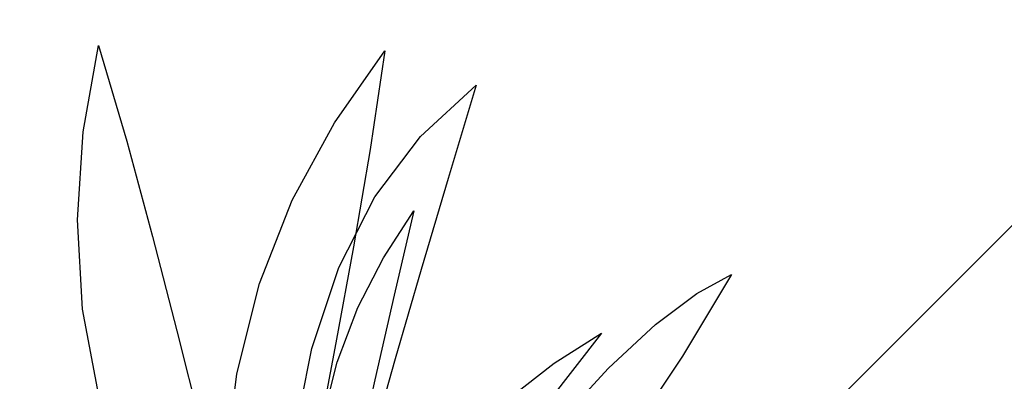
# Model space of a CAD drawing. Units: inches. Extents: x 3590 to 5167, y 65 to 1917.
# Tile 53 of 100: x 4947.17 to 4967.82, y 1530.53 to 1538.11. Entities that reach past the tile are written whole.
import ezdxf

# ---------------------------------------------------------------- set-up
doc = ezdxf.new("R2010")
doc.units = ezdxf.units.IN
doc.layers.add('A-FLOR-PATT', color=8, linetype='Continuous', lineweight=13)
doc.layers.add('L-PLNT', color=94, linetype='Continuous', lineweight=18)
doc.layers.add('DIENHOA', color=3, linetype='Continuous')

# ---------------------------------------------------------------- blocks, each defined once
blk = doc.blocks.new('Cay03_mb')
at = {"layer": 'DIENHOA'}
for p, q in [((118.58, 555.3), (166.15, 599.14)), ((166.15, 599.14), (142.15, 519.35)), ((79.49, 503.68), (118.58, 555.3)), ((142.15, 519.35), (118.96, 441.66)), ((48.56, 443.58), (79.49, 503.68)), ((25.49, 374.33), (48.56, 443.58)), ((118.96, 441.66), (96.72, 365.58)), ((9.94, 295.25), (25.49, 374.33)), ((96.72, 365.58), (75.6, 290.61))]:
    blk.add_line(p, q, dxfattribs=at)
for points in [[(23.69, -5.44), (-41, 82.2), (-91.83, 167.08), (-129.72, 249.45), (-155.55, 329.59), (-170.25, 407.76), (-174.71, 484.23), (-169.84, 559.26), (-156.54, 633.12)], [(-156.54, 633.12), (-132.46, 551.33), (-110.51, 470.02), (-89.84, 389.22), (-69.62, 308.98), (-48.99, 229.35), (-27.13, 150.38), (-3.18, 72.1), (23.69, -5.44)], [(-16.39, -26.73), (-38.34, 79.96), (-48.88, 178.33), (-48.7, 269), (-38.53, 352.58), (-19.08, 429.71), (8.95, 500.99), (44.86, 567.06), (87.92, 628.52)], [(87.92, 628.52), (75.46, 544.18), (61.27, 461.15), (46.13, 379.14), (30.83, 297.82), (16.14, 216.89), (2.85, 136.03), (-8.25, 54.92), (-16.39, -26.73)], [(23.69, -5.44), (19.84, 92.99), (20.28, 176.97), (25.02, 248.55), (34.03, 309.77), (47.33, 362.68), (64.91, 409.31), (86.75, 451.72), (112.87, 491.95)], [(112.87, 491.95), (95.99, 419.69), (79.46, 347.37), (63.92, 276.46), (50.01, 208.43), (38.38, 144.75), (29.69, 86.9), (24.57, 36.35), (23.69, -5.44)], [(384.28, 437.45), (342.25, 367.83), (298.14, 301.71), (252.56, 239.37), (206.11, 181.11), (159.39, 127.21), (113.01, 77.96), (67.57, 33.64), (23.69, -5.44)], [(23.69, -5.44), (79.88, 91.71), (134.12, 176.21), (185.81, 248.4), (234.31, 308.65), (279.02, 357.33), (319.33, 394.78), (354.62, 421.37), (384.28, 437.45)], [(273.24, 387.35), (227.6, 328.83), (182.25, 270.12), (138.39, 212.28), (97.23, 156.36), (59.96, 103.43), (27.8, 54.57), (1.94, 10.82), (-16.39, -26.73)], [(-16.39, -26.73), (21.41, 64.22), (57.05, 140.27), (91.37, 203.26), (125.24, 255.05), (159.51, 297.5), (195.03, 332.46), (232.65, 361.79), (273.24, 387.35)]]:
    blk.add_lwpolyline(points, dxfattribs=at)

msp = doc.modelspace()

# ---------------------------------------------------------------- hatches: boundary and pattern name
at = {"layer": 'A-FLOR-PATT', "transparency": 33554687}
h = msp.add_hatch(dxfattribs=at)
h.set_pattern_fill('AR-HBONE', color=256, scale=0.2)
h.set_pattern_definition([(45, (-588.972, 0), (0, 28.73682), [60.96, -20.32]), (135, (-574.604, 14.368), (3e-15, 28.73682), [60.96, -20.32])])
h.paths.add_polyline_path([(5071.274, 1796.999), (4933.274, 1796.999), (4933.274, 1753.999), (4962.774, 1753.999, -0.414214), (4928.774, 1719.999), (4933.274, 1718.999), (4933.274, 1334.999), (5071.274, 1334.999)])
h.paths.add_polyline_path([(4951.78, 1521.077), (4951.715, 1521.04), (4951.563, 1520.895)], flags=16)
h.paths.add_polyline_path([(4952.267, 1521.376), (4952.198, 1521.371), (4952.198, 1521.356)], flags=0)
h.paths.add_polyline_path([(4967.051, 1529.728), (4965.231, 1528.694), (4963.411, 1527.714), (4961.756, 1526.851), (4963.589, 1527.449), (4964.036, 1527.478), (4962.975, 1527.249), (4961.76, 1526.852), (4959.792, 1525.834), (4958.005, 1524.895), (4956.24, 1523.93), (4954.504, 1522.919), (4954.129, 1522.682), (4953.361, 1521.997), (4953.366, 1521.998), (4953.605, 1522.064), (4955.106, 1522.761), (4956.921, 1523.434), (4958.678, 1523.915), (4960.358, 1524.2), (4961.945, 1524.286), (4964.171, 1524.108), (4965.958, 1523.309), (4963.863, 1522.976), (4965.187, 1522.499), (4963.366, 1522.497), (4961.545, 1522.487), (4959.764, 1522.461), (4958.304, 1522.419), (4957.974, 1522.388), (4956.307, 1522.232), (4954.718, 1522.071), (4953.251, 1521.899), (4953.525, 1521.623), (4954.331, 1521.379), (4956.243, 1521.23), (4958.039, 1520.93), (4959.684, 1520.483), (4961.16, 1519.896), (4963.107, 1518.8), (4964.393, 1517.325), (4962.973, 1517.726), (4964.558, 1516.661), (4965.407, 1515.708), (4963.507, 1516.322), (4961.68, 1517.005), (4959.935, 1517.745), (4958.282, 1518.528), (4956.732, 1519.343), (4955.295, 1520.175), (4954.672, 1520.572), (4954.513, 1520.627), (4955.658, 1519.318), (4956.703, 1517.982), (4957.644, 1516.647), (4958.485, 1515.334), (4959.55, 1513.524), (4960.438, 1511.769), (4958.841, 1513.62), (4957.452, 1515.325), (4955.819, 1517.459), (4956.665, 1515.448), (4957.111, 1513.923), (4957.447, 1511.714), (4957.076, 1509.793), (4956.538, 1511.11), (4955.992, 1512.569), (4955.444, 1514.125), (4954.898, 1515.735), (4954.357, 1517.356), (4953.824, 1518.943), (4953.305, 1520.452), (4953.065, 1521.116), (4952.971, 1521.146), (4952.949, 1521.086), (4952.73, 1520.199), (4953.37, 1518.024), (4953.757, 1516.373), (4954.051, 1514.765), (4954.264, 1513.221), (4954.471, 1511.131), (4954.497, 1510.402), (4954.409, 1511.76), (4954.264, 1513.221), (4954.051, 1514.765), (4953.757, 1516.373), (4953.37, 1518.024), (4952.877, 1519.698), (4952.716, 1520.141), (4952.533, 1519.059), (4952.374, 1517.789), (4952.219, 1516.312), (4952.046, 1514.6), (4951.833, 1512.626), (4951.557, 1510.363), (4951.203, 1512.168), (4950.852, 1514.339), (4950.985, 1516.376), (4951.66, 1518.286), (4952.593, 1520.481), (4952.357, 1521.13), (4951.855, 1520.328), (4950.839, 1518.908), (4949.777, 1517.587), (4948.916, 1516.617), (4948.111, 1515.256), (4947.089, 1513.554), (4945.889, 1511.615), (4946.326, 1513.402), (4946.562, 1514.249), (4945.528, 1513.327), (4944.581, 1512.531), (4946.018, 1514.508), (4947.204, 1516.048), (4947.893, 1517.313), (4949.307, 1518.764), (4950.414, 1519.767), (4950.451, 1519.806), (4952.267, 1521.376), (4951.645, 1521.493), (4950.404, 1521.18), (4948.044, 1520.359), (4946.119, 1519.452), (4944.572, 1518.475), (4943.35, 1517.443), (4941.997, 1515.92), (4941.661, 1515.275), (4942.813, 1516.99), (4944.572, 1518.475), (4946.119, 1519.452), (4948.044, 1520.359), (4950.404, 1521.18), (4951.645, 1521.493), (4949.647, 1521.868), (4948.6, 1521.756), (4947.126, 1521.57), (4945.42, 1521.348), (4943.45, 1521.105), (4941.183, 1520.856), (4942.86, 1521.613), (4943.873, 1522.03), (4942.952, 1521.909), (4941.41, 1521.485), (4939.543, 1520.67), (4938.968, 1520.226), (4940.733, 1521.299), (4942.952, 1521.909), (4943.702, 1522.008), (4945.894, 1522.7), (4947.565, 1522.714), (4948.921, 1522.566), (4951.131, 1522.183), (4950.971, 1522.297), (4948.129, 1523.006), (4946.035, 1523.707), (4944.232, 1524.521), (4942.707, 1525.461), (4941.444, 1526.537), (4940.43, 1527.761), (4939.649, 1529.143), (4941.421, 1528.122), (4943.147, 1527.132), (4944.841, 1526.175), (4946.514, 1525.25), (4948.179, 1524.359), (4948.365, 1524.263), (4946.475, 1526.045), (4945.181, 1527.54), (4944.19, 1529.033), (4943.496, 1530.54), (4943.278, 1531.36), (4942.498, 1531.919), (4943.114, 1531.762), (4942.959, 1533.659), (4944.14, 1531.989), (4944.612, 1531.323), (4946.202, 1530.463), (4947.486, 1529.509), (4948.79, 1528.226), (4950.368, 1526.237), (4949.485, 1528.155), (4948.851, 1530.123), (4948.491, 1532.041), (4948.381, 1533.918), (4948.501, 1535.76), (4948.827, 1537.573), (4949.418, 1535.565), (4949.957, 1533.569), (4950.464, 1531.586), (4950.961, 1529.617), (4951.391, 1527.954), (4951.724, 1530.687), (4952.201, 1532.58), (4952.889, 1534.33), (4953.77, 1535.951), (4954.827, 1537.46), (4954.521, 1535.39), (4954.273, 1533.937), (4955.58, 1535.663), (4956.748, 1536.739), (4956.159, 1534.78), (4955.589, 1532.873), (4955.043, 1531.006), (4954.525, 1529.166), (4954.038, 1527.341), (4953.638, 1525.733), (4953.611, 1525.586), (4953.398, 1524.166), (4953.382, 1524.009), (4954.07, 1525.476), (4954.912, 1527.022), (4956.136, 1528.894), (4957.847, 1530.577), (4959.376, 1531.54), (4958.256, 1530.104), (4957.143, 1528.663), (4956.066, 1527.243), (4955.056, 1525.871), (4954.141, 1524.571), (4953.352, 1523.372), (4953.311, 1523.303), (4953.273, 1522.925), (4953.261, 1522.382), (4954.103, 1523.373), (4954.63, 1524.284), (4955.961, 1526.358), (4957.23, 1528.13), (4958.421, 1529.609), (4960.037, 1531.368), (4961.374, 1532.375), (4962.101, 1532.77), (4961.07, 1531.061), (4959.987, 1529.438), (4958.869, 1527.908), (4958.15, 1527.007), (4959.803, 1528.003), (4961.589, 1528.793), (4963.391, 1529.328), (4965.211, 1529.632)], flags=16)
h.paths.add_polyline_path([(4962.944, 1523.182), (4961.107, 1523.422), (4960.392, 1523.362), (4962.35, 1523.331)], flags=0)
h.paths.add_polyline_path([(5049.541, 1584.551), (5049.476, 1584.515), (5049.325, 1584.37)], flags=16)
h.paths.add_polyline_path([(5050.028, 1584.851), (5049.959, 1584.845), (5049.959, 1584.83)], flags=0)
h.paths.add_polyline_path([(5042.333, 1581.949), (5043.88, 1582.926), (5045.806, 1583.833), (5048.165, 1584.654), (5049.406, 1584.967), (5047.408, 1585.342), (5046.361, 1585.231), (5044.888, 1585.044), (5043.181, 1584.822), (5041.211, 1584.579), (5038.944, 1584.33), (5040.622, 1585.087), (5041.634, 1585.504), (5040.713, 1585.383), (5039.171, 1584.959), (5037.304, 1584.144), (5036.729, 1583.7), (5038.494, 1584.773), (5040.713, 1585.383), (5041.463, 1585.482), (5043.655, 1586.174), (5045.326, 1586.188), (5046.682, 1586.04), (5048.893, 1585.657), (5048.732, 1585.771), (5045.891, 1586.48), (5043.796, 1587.181), (5041.994, 1587.996), (5040.468, 1588.935), (5039.205, 1590.011), (5038.191, 1591.235), (5037.41, 1592.617), (5039.182, 1591.596), (5040.909, 1590.607), (5042.602, 1589.649), (5044.275, 1588.724), (5045.94, 1587.833), (5046.126, 1587.738), (5044.237, 1589.519), (5042.942, 1591.015), (5041.952, 1592.508), (5041.257, 1594.014), (5041.039, 1594.834), (5040.26, 1595.393), (5040.875, 1595.237), (5040.721, 1597.133), (5041.901, 1595.463), (5042.373, 1594.798), (5043.963, 1593.938), (5045.247, 1592.983), (5046.552, 1591.701), (5048.129, 1589.712), (5047.247, 1591.63), (5046.613, 1593.597), (5046.252, 1595.515), (5046.142, 1597.392), (5046.262, 1599.234), (5046.588, 1601.047), (5047.179, 1599.039), (5047.718, 1597.043), (5048.225, 1595.06), (5048.722, 1593.091), (5049.152, 1591.429), (5049.485, 1594.161), (5049.962, 1596.054), (5050.65, 1597.804), (5051.532, 1599.425), (5052.589, 1600.934), (5052.283, 1598.864), (5052.034, 1597.411), (5053.341, 1599.137), (5054.509, 1600.213), (5053.92, 1598.254), (5053.35, 1596.348), (5052.805, 1594.48), (5052.286, 1592.64), (5051.799, 1590.815), (5051.4, 1589.207), (5051.373, 1589.06), (5051.159, 1587.64), (5051.143, 1587.483), (5051.831, 1588.95), (5052.673, 1590.496), (5053.898, 1592.368), (5055.608, 1594.051), (5057.137, 1595.014), (5056.017, 1593.578), (5054.904, 1592.137), (5053.828, 1590.717), (5052.817, 1589.345), (5051.902, 1588.046), (5051.113, 1586.846), (5051.072, 1586.777), (5051.034, 1586.399), (5051.022, 1585.856), (5051.864, 1586.847), (5052.391, 1587.758), (5053.723, 1589.832), (5054.991, 1591.604), (5056.182, 1593.083), (5057.798, 1594.842), (5059.135, 1595.849), (5059.863, 1596.244), (5058.831, 1594.535), (5057.749, 1592.912), (5056.63, 1591.382), (5055.912, 1590.482), (5057.564, 1591.477), (5059.35, 1592.267), (5061.152, 1592.802), (5062.972, 1593.106), (5064.812, 1593.203), (5062.992, 1592.169), (5061.172, 1591.188), (5059.518, 1590.325), (5061.35, 1590.924), (5061.797, 1590.952), (5060.737, 1590.723), (5059.521, 1590.326), (5057.553, 1589.308), (5055.766, 1588.369), (5054.002, 1587.404), (5052.265, 1586.393), (5051.891, 1586.156), (5051.122, 1585.471), (5051.127, 1585.472), (5051.366, 1585.538), (5052.867, 1586.235), (5054.682, 1586.908), (5056.439, 1587.389), (5058.12, 1587.675), (5059.706, 1587.76), (5061.933, 1587.583), (5063.719, 1586.783), (5061.624, 1586.45), (5062.949, 1585.973), (5061.127, 1585.971), (5059.307, 1585.961), (5057.525, 1585.935), (5056.065, 1585.893), (5055.735, 1585.862), (5054.068, 1585.707), (5052.479, 1585.546), (5051.012, 1585.373), (5051.286, 1585.097), (5052.092, 1584.853), (5054.004, 1584.704), (5055.8, 1584.404), (5057.446, 1583.958), (5058.921, 1583.37), (5060.868, 1582.274), (5062.154, 1580.799), (5060.734, 1581.2), (5062.32, 1580.135), (5063.168, 1579.182), (5061.269, 1579.796), (5059.441, 1580.479), (5057.696, 1581.219), (5056.043, 1582.003), (5054.493, 1582.817), (5053.057, 1583.649), (5052.433, 1584.047), (5052.274, 1584.101), (5053.42, 1582.793), (5054.464, 1581.457), (5055.405, 1580.121), (5056.247, 1578.809), (5057.311, 1576.998), (5058.199, 1575.244), (5056.602, 1577.094), (5055.213, 1578.799), (5053.58, 1580.933), (5054.427, 1578.922), (5054.872, 1577.397), (5055.208, 1575.189), (5054.838, 1573.267), (5054.299, 1574.584), (5053.754, 1576.043), (5053.206, 1577.599), (5052.659, 1579.209), (5052.118, 1580.83), (5051.585, 1582.417), (5051.066, 1583.927), (5050.826, 1584.59), (5050.733, 1584.62), (5050.711, 1584.561), (5050.491, 1583.673), (5051.131, 1581.498), (5051.518, 1579.847), (5051.813, 1578.24), (5052.026, 1576.695), (5052.233, 1574.605), (5052.258, 1573.876), (5052.17, 1575.234), (5052.026, 1576.695), (5051.813, 1578.24), (5051.518, 1579.847), (5051.131, 1581.498), (5050.638, 1583.172), (5050.477, 1583.615), (5050.294, 1582.533), (5050.136, 1581.263), (5049.981, 1579.786), (5049.807, 1578.074), (5049.594, 1576.1), (5049.318, 1573.837), (5048.965, 1575.642), (5048.613, 1577.813), (5048.747, 1579.85), (5049.421, 1581.76), (5050.354, 1583.955), (5050.118, 1584.604), (5049.616, 1583.802), (5048.6, 1582.382), (5047.538, 1581.061), (5046.677, 1580.091), (5045.872, 1578.73), (5044.85, 1577.028), (5043.651, 1575.089), (5044.087, 1576.877), (5044.324, 1577.723), (5043.289, 1576.801), (5042.342, 1576.005), (5043.779, 1577.982), (5044.966, 1579.522), (5045.655, 1580.787), (5047.068, 1582.239), (5048.175, 1583.241), (5048.213, 1583.28), (5050.028, 1584.851), (5049.406, 1584.967), (5048.165, 1584.654), (5045.806, 1583.833), (5043.88, 1582.926), (5042.333, 1581.949), (5041.111, 1580.917), (5039.758, 1579.394), (5039.423, 1578.749), (5040.575, 1580.464)], flags=16)
h.paths.add_polyline_path([(4954.799, 1533.12), (4954.262, 1532.079), (4953.831, 1530.935), (4953.505, 1529.636), (4953.283, 1528.133), (4953.167, 1526.376), (4953.156, 1524.315), (4953.277, 1521.236), (4952.802, 1521.842), (4951.557, 1521.998), (4950.976, 1521.961), (4952.661, 1521.941), (4952.802, 1521.842), (4953.152, 1523.593), (4953.167, 1526.376), (4953.283, 1528.133), (4953.609, 1530.346), (4954.456, 1532.592)], flags=0)
h.paths.add_polyline_path([(5050.563, 1585.316), (5049.318, 1585.472), (5048.737, 1585.435), (5050.422, 1585.415), (5050.563, 1585.316), (5050.914, 1587.067), (5050.928, 1589.851), (5051.045, 1591.607), (5051.371, 1593.82), (5052.217, 1596.066), (5052.56, 1596.594), (5052.024, 1595.554), (5051.592, 1594.409), (5051.266, 1593.11), (5051.045, 1591.607), (5050.928, 1589.851), (5050.918, 1587.789), (5051.038, 1584.71)], flags=0)
h.paths.add_polyline_path([(5058.153, 1586.836), (5060.111, 1586.805), (5060.705, 1586.656), (5058.868, 1586.896)], flags=0)
h.paths.add_polyline_path([(5049.541, 1430.936), (5049.476, 1430.9), (5049.325, 1430.755)], flags=16)
h.paths.add_polyline_path([(5050.028, 1431.236), (5049.959, 1431.231), (5049.959, 1431.215)], flags=0)
h.paths.add_polyline_path([(5046.588, 1447.432), (5047.179, 1445.425), (5047.718, 1443.429), (5048.225, 1441.446), (5048.722, 1439.476), (5049.152, 1437.814), (5049.485, 1440.546), (5049.962, 1442.439), (5050.65, 1444.189), (5051.532, 1445.811), (5052.589, 1447.319), (5052.283, 1445.249), (5052.034, 1443.796), (5053.341, 1445.522), (5054.509, 1446.598), (5053.92, 1444.64), (5053.35, 1442.733), (5052.805, 1440.865), (5052.286, 1439.025), (5051.799, 1437.201), (5051.4, 1435.592), (5051.373, 1435.445), (5051.159, 1434.025), (5051.143, 1433.868), (5051.831, 1435.335), (5052.673, 1436.881), (5053.898, 1438.753), (5055.608, 1440.436), (5057.137, 1441.4), (5056.017, 1439.963), (5054.904, 1438.522), (5053.828, 1437.102), (5052.817, 1435.73), (5051.902, 1434.431), (5051.113, 1433.231), (5051.072, 1433.162), (5051.034, 1432.784), (5051.022, 1432.242), (5051.864, 1433.232), (5052.391, 1434.143), (5053.723, 1436.217), (5054.991, 1437.989), (5056.182, 1439.468), (5057.798, 1441.227), (5059.135, 1442.235), (5059.863, 1442.629), (5058.831, 1440.921), (5057.749, 1439.298), (5056.63, 1437.767), (5055.912, 1436.867), (5057.564, 1437.863), (5059.35, 1438.652), (5061.152, 1439.187), (5062.972, 1439.491), (5064.812, 1439.588), (5062.992, 1438.554), (5061.172, 1437.573), (5059.518, 1436.71), (5061.35, 1437.309), (5061.797, 1437.337), (5060.737, 1437.108), (5059.521, 1436.711), (5057.553, 1435.693), (5055.766, 1434.754), (5054.002, 1433.789), (5052.265, 1432.778), (5051.891, 1432.541), (5051.122, 1431.856), (5051.127, 1431.857), (5051.366, 1431.923), (5052.867, 1432.62), (5054.682, 1433.293), (5056.439, 1433.775), (5058.12, 1434.06), (5059.706, 1434.145), (5061.933, 1433.968), (5063.719, 1433.168), (5061.624, 1432.835), (5062.949, 1432.358), (5061.127, 1432.357), (5059.307, 1432.346), (5057.525, 1432.32), (5056.065, 1432.278), (5055.735, 1432.248), (5054.068, 1432.092), (5052.479, 1431.931), (5051.012, 1431.759), (5051.286, 1431.482), (5052.092, 1431.238), (5054.004, 1431.089), (5055.8, 1430.789), (5057.446, 1430.343), (5058.921, 1429.755), (5060.868, 1428.66), (5062.154, 1427.185), (5060.734, 1427.585), (5062.32, 1426.52), (5063.168, 1425.567), (5061.269, 1426.181), (5059.441, 1426.865), (5057.696, 1427.604), (5056.043, 1428.388), (5054.493, 1429.202), (5053.057, 1430.034), (5052.433, 1430.432), (5052.274, 1430.487), (5053.42, 1429.178), (5054.464, 1427.842), (5055.405, 1426.506), (5056.247, 1425.194), (5057.311, 1423.383), (5058.199, 1421.629), (5056.602, 1423.479), (5055.213, 1425.184), (5053.58, 1427.318), (5054.427, 1425.307), (5054.872, 1423.782), (5055.208, 1421.574), (5054.838, 1419.652), (5054.299, 1420.97), (5053.754, 1422.428), (5053.206, 1423.984), (5052.659, 1425.595), (5052.118, 1427.215), (5051.585, 1428.802), (5051.066, 1430.312), (5050.826, 1430.975), (5050.733, 1431.005), (5050.711, 1430.946), (5050.491, 1430.058), (5051.131, 1427.883), (5051.518, 1426.232), (5051.813, 1424.625), (5052.026, 1423.081), (5052.233, 1420.991), (5052.258, 1420.261), (5052.17, 1421.619), (5052.026, 1423.081), (5051.813, 1424.625), (5051.518, 1426.232), (5051.131, 1427.883), (5050.638, 1429.558), (5050.477, 1430.001), (5050.294, 1428.918), (5050.136, 1427.648), (5049.981, 1426.171), (5049.807, 1424.459), (5049.594, 1422.485), (5049.318, 1420.222), (5048.965, 1422.028), (5048.613, 1424.199), (5048.747, 1426.235), (5049.421, 1428.146), (5050.354, 1430.34), (5050.118, 1430.989), (5049.616, 1430.187), (5048.6, 1428.768), (5047.538, 1427.446), (5046.677, 1426.477), (5045.872, 1425.116), (5044.85, 1423.413), (5043.651, 1421.474), (5044.087, 1423.262), (5044.324, 1424.109), (5043.289, 1423.186), (5042.342, 1422.391), (5043.779, 1424.368), (5044.966, 1425.907), (5045.655, 1427.173), (5047.068, 1428.624), (5048.175, 1429.627), (5048.213, 1429.666), (5050.028, 1431.236), (5049.406, 1431.353), (5048.165, 1431.039), (5045.806, 1430.218), (5043.88, 1429.311), (5042.333, 1428.334), (5041.111, 1427.302), (5039.758, 1425.779), (5039.423, 1425.134), (5040.575, 1426.849), (5042.333, 1428.334), (5043.88, 1429.311), (5045.806, 1430.218), (5048.165, 1431.039), (5049.406, 1431.353), (5047.408, 1431.727), (5046.361, 1431.616), (5044.888, 1431.429), (5043.181, 1431.207), (5041.211, 1430.964), (5038.944, 1430.715), (5040.622, 1431.472), (5041.634, 1431.89), (5040.713, 1431.769), (5039.171, 1431.345), (5037.304, 1430.53), (5036.729, 1430.085), (5038.494, 1431.158), (5040.713, 1431.769), (5041.463, 1431.867), (5043.655, 1432.559), (5045.326, 1432.573), (5046.682, 1432.425), (5048.893, 1432.042), (5048.732, 1432.156), (5045.891, 1432.865), (5043.796, 1433.566), (5041.994, 1434.381), (5040.468, 1435.321), (5039.205, 1436.396), (5038.191, 1437.62), (5037.41, 1439.002), (5039.182, 1437.982), (5040.909, 1436.992), (5042.602, 1436.034), (5044.275, 1435.109), (5045.94, 1434.218), (5046.126, 1434.123), (5044.237, 1435.904), (5042.942, 1437.4), (5041.952, 1438.893), (5041.257, 1440.399), (5041.039, 1441.219), (5040.26, 1441.778), (5040.875, 1441.622), (5040.721, 1443.518), (5041.901, 1441.848), (5042.373, 1441.183), (5043.963, 1440.323), (5045.247, 1439.369), (5046.552, 1438.086), (5048.129, 1436.097), (5047.247, 1438.015), (5046.613, 1439.982), (5046.252, 1441.901), (5046.142, 1443.778), (5046.262, 1445.619)], flags=16)
h.paths.add_polyline_path([(5052.382, 1444.255), (5051.623, 1442.78), (5052.024, 1441.939), (5052.56, 1442.98)], flags=0)
h.paths.add_polyline_path([(5050.563, 1431.701), (5049.318, 1431.857), (5048.737, 1431.821), (5050.422, 1431.8)], flags=0)
h.paths.add_polyline_path([(5058.153, 1433.221), (5060.111, 1433.19), (5060.705, 1433.041), (5058.868, 1433.281)], flags=0)
h.paths.add_polyline_path([(5049.541, 1352.285), (5049.476, 1352.249), (5049.325, 1352.104)], flags=16)
h.paths.add_polyline_path([(5050.028, 1352.585), (5049.959, 1352.58), (5049.959, 1352.564)], flags=0)
h.paths.add_polyline_path([(5046.588, 1368.781), (5047.179, 1366.774), (5047.718, 1364.778), (5048.225, 1362.795), (5048.722, 1360.825), (5049.152, 1359.163), (5049.485, 1361.896), (5049.962, 1363.789), (5050.65, 1365.538), (5051.532, 1367.16), (5052.589, 1368.669), (5052.283, 1366.598), (5052.034, 1365.145), (5053.341, 1366.871), (5054.509, 1367.947), (5053.92, 1365.989), (5053.35, 1364.082), (5052.805, 1362.214), (5052.286, 1360.374), (5051.799, 1358.55), (5051.4, 1356.942), (5051.373, 1356.794), (5051.159, 1355.374), (5051.143, 1355.218), (5051.831, 1356.684), (5052.673, 1358.23), (5053.898, 1360.102), (5055.608, 1361.786), (5057.137, 1362.749), (5056.017, 1361.313), (5054.904, 1359.872), (5053.828, 1358.452), (5052.817, 1357.079), (5051.902, 1355.78), (5051.113, 1354.581), (5051.072, 1354.512), (5051.034, 1354.133), (5051.022, 1353.591), (5051.864, 1354.581), (5052.391, 1355.492), (5053.723, 1357.566), (5054.991, 1359.338), (5056.182, 1360.817), (5057.798, 1362.577), (5059.135, 1363.584), (5059.863, 1363.979), (5058.831, 1362.27), (5057.749, 1360.647), (5056.63, 1359.117), (5055.912, 1358.216), (5057.564, 1359.212), (5059.35, 1360.001), (5061.152, 1360.536), (5062.972, 1360.841), (5064.812, 1360.937), (5062.992, 1359.903), (5061.172, 1358.923), (5059.518, 1358.059), (5061.35, 1358.658), (5061.797, 1358.687), (5060.737, 1358.458), (5059.521, 1358.061), (5057.553, 1357.043), (5055.766, 1356.103), (5054.002, 1355.138), (5052.265, 1354.127), (5051.891, 1353.89), (5051.122, 1353.206), (5051.127, 1353.206), (5051.366, 1353.272), (5052.867, 1353.969), (5054.682, 1354.643), (5056.439, 1355.124), (5058.12, 1355.409), (5059.706, 1355.495), (5061.933, 1355.317), (5063.719, 1354.518), (5061.624, 1354.184), (5062.949, 1353.708), (5061.127, 1353.706), (5059.307, 1353.695), (5057.525, 1353.669), (5056.065, 1353.627), (5055.735, 1353.597), (5054.068, 1353.441), (5052.479, 1353.28), (5051.012, 1353.108), (5051.286, 1352.831), (5052.092, 1352.587), (5054.004, 1352.439), (5055.8, 1352.138), (5057.446, 1351.692), (5058.921, 1351.104), (5060.868, 1350.009), (5062.154, 1348.534), (5060.734, 1348.935), (5062.32, 1347.869), (5063.168, 1346.916), (5061.269, 1347.53), (5059.441, 1348.214), (5057.696, 1348.954), (5056.043, 1349.737), (5054.493, 1350.551), (5053.057, 1351.383), (5052.433, 1351.781), (5052.274, 1351.836), (5053.42, 1350.527), (5054.464, 1349.191), (5055.405, 1347.855), (5056.247, 1346.543), (5057.311, 1344.733), (5058.199, 1342.978), (5056.602, 1344.828), (5055.213, 1346.534), (5053.58, 1348.667), (5054.427, 1346.656), (5054.872, 1345.132), (5055.208, 1342.923), (5054.838, 1341.002), (5054.299, 1342.319), (5053.754, 1343.778), (5053.206, 1345.334), (5052.659, 1346.944), (5052.118, 1348.564), (5051.585, 1350.151), (5051.066, 1351.661), (5050.826, 1352.324), (5050.733, 1352.355), (5050.711, 1352.295), (5050.491, 1351.408), (5051.131, 1349.232), (5051.518, 1347.581), (5051.813, 1345.974), (5052.026, 1344.43), (5052.233, 1342.34), (5052.258, 1341.61), (5052.17, 1342.969), (5052.026, 1344.43), (5051.813, 1345.974), (5051.518, 1347.581), (5051.131, 1349.232), (5050.638, 1350.907), (5050.477, 1351.35), (5050.294, 1350.267), (5050.136, 1348.997), (5049.981, 1347.52), (5049.807, 1345.809), (5049.594, 1343.835), (5049.318, 1341.571), (5048.965, 1343.377), (5048.613, 1345.548), (5048.747, 1347.585), (5049.421, 1349.495), (5050.354, 1351.689), (5050.118, 1352.339), (5049.616, 1351.536), (5048.6, 1350.117), (5047.538, 1348.795), (5046.677, 1347.826), (5045.872, 1346.465), (5044.85, 1344.763), (5043.651, 1342.824), (5044.087, 1344.611), (5044.324, 1345.458), (5043.289, 1344.535), (5042.342, 1343.74), (5043.779, 1345.717), (5044.966, 1347.256), (5045.655, 1348.522), (5047.068, 1349.973), (5048.175, 1350.976), (5048.213, 1351.015), (5050.028, 1352.585), (5049.406, 1352.702), (5048.165, 1352.388), (5045.806, 1351.567), (5043.88, 1350.661), (5042.333, 1349.683), (5041.111, 1348.651), (5039.758, 1347.128), (5039.423, 1346.483), (5040.575, 1348.198), (5042.333, 1349.683), (5043.88, 1350.661), (5045.806, 1351.567), (5048.165, 1352.388), (5049.406, 1352.702), (5047.408, 1353.076), (5046.361, 1352.965), (5044.888, 1352.779), (5043.181, 1352.556), (5041.211, 1352.313), (5038.944, 1352.065), (5040.622, 1352.821), (5041.634, 1353.239), (5040.713, 1353.118), (5039.171, 1352.694), (5037.304, 1351.879), (5036.729, 1351.434), (5038.494, 1352.508), (5040.713, 1353.118), (5041.463, 1353.216), (5043.655, 1353.909), (5045.326, 1353.923), (5046.682, 1353.774), (5048.893, 1353.391), (5048.732, 1353.506), (5045.891, 1354.214), (5043.796, 1354.915), (5041.994, 1355.73), (5040.468, 1356.67), (5039.205, 1357.746), (5038.191, 1358.969), (5037.41, 1360.352), (5039.182, 1359.331), (5040.909, 1358.341), (5042.602, 1357.383), (5044.275, 1356.458), (5045.94, 1355.567), (5046.126, 1355.472), (5044.237, 1357.253), (5042.942, 1358.749), (5041.952, 1360.242), (5041.257, 1361.748), (5041.039, 1362.568), (5040.26, 1363.128), (5040.875, 1362.971), (5040.721, 1364.867), (5041.901, 1363.197), (5042.373, 1362.532), (5043.963, 1361.672), (5045.247, 1360.718), (5046.552, 1359.435), (5048.129, 1357.446), (5047.247, 1359.364), (5046.613, 1361.331), (5046.252, 1363.25), (5046.142, 1365.127), (5046.262, 1366.969)], flags=16)
h.paths.add_polyline_path([(5052.382, 1365.604), (5051.623, 1364.129), (5052.024, 1363.288), (5052.56, 1364.329)], flags=0)
h.paths.add_polyline_path([(4951.78, 1698.041), (4951.715, 1698.005), (4951.563, 1697.859)], flags=16)
h.paths.add_polyline_path([(4952.267, 1698.341), (4952.198, 1698.335), (4952.198, 1698.32)], flags=0)
h.paths.add_polyline_path([(4957.076, 1686.757), (4956.538, 1688.074), (4955.992, 1689.533), (4955.444, 1691.089), (4954.898, 1692.699), (4954.357, 1694.32), (4953.824, 1695.907), (4953.305, 1697.417), (4953.065, 1698.08), (4952.971, 1698.11), (4952.949, 1698.051), (4952.73, 1697.163), (4953.37, 1694.988), (4953.757, 1693.337), (4954.051, 1691.729), (4954.264, 1690.185), (4954.471, 1688.095), (4954.497, 1687.366), (4954.409, 1688.724), (4954.264, 1690.185), (4954.051, 1691.729), (4953.757, 1693.337), (4953.37, 1694.988), (4952.877, 1696.662), (4952.716, 1697.105), (4952.533, 1696.023), (4952.374, 1694.753), (4952.219, 1693.276), (4952.046, 1691.564), (4951.833, 1689.59), (4951.557, 1687.327), (4951.203, 1689.132), (4950.852, 1691.303), (4950.985, 1693.34), (4951.66, 1695.25), (4952.593, 1697.445), (4952.357, 1698.094), (4951.855, 1697.292), (4950.839, 1695.872), (4949.777, 1694.551), (4948.916, 1693.581), (4948.111, 1692.22), (4947.089, 1690.518), (4945.889, 1688.579), (4946.326, 1690.366), (4946.562, 1691.213), (4945.528, 1690.291), (4944.581, 1689.495), (4946.018, 1691.472), (4947.204, 1693.012), (4947.893, 1694.277), (4949.307, 1695.729), (4950.414, 1696.731), (4950.451, 1696.77), (4952.267, 1698.341), (4951.645, 1698.457), (4950.404, 1698.144), (4948.044, 1697.323), (4946.119, 1696.416), (4944.572, 1695.439), (4943.35, 1694.407), (4941.997, 1692.884), (4941.661, 1692.239), (4942.813, 1693.954), (4944.572, 1695.439), (4946.119, 1696.416), (4948.044, 1697.323), (4950.404, 1698.144), (4951.645, 1698.457), (4949.647, 1698.832), (4948.6, 1698.72), (4947.126, 1698.534), (4945.42, 1698.312), (4943.45, 1698.069), (4941.183, 1697.82), (4942.86, 1698.577), (4943.873, 1698.994), (4942.952, 1698.873), (4941.41, 1698.449), (4939.543, 1697.634), (4938.968, 1697.19), (4940.733, 1698.263), (4942.952, 1698.873), (4943.702, 1698.972), (4945.894, 1699.664), (4947.565, 1699.678), (4948.921, 1699.53), (4951.131, 1699.147), (4950.971, 1699.261), (4948.129, 1699.97), (4946.035, 1700.671), (4944.232, 1701.486), (4942.707, 1702.425), (4941.444, 1703.501), (4940.43, 1704.725), (4939.649, 1706.107), (4941.421, 1705.086), (4943.147, 1704.097), (4944.841, 1703.139), (4946.514, 1702.214), (4948.179, 1701.323), (4948.365, 1701.227), (4946.475, 1703.009), (4945.181, 1704.505), (4944.19, 1705.997), (4943.496, 1707.504), (4943.278, 1708.324), (4942.498, 1708.883), (4943.114, 1708.727), (4942.959, 1710.623), (4944.14, 1708.953), (4944.612, 1708.287), (4946.202, 1707.428), (4947.486, 1706.473), (4948.79, 1705.191), (4950.368, 1703.202), (4949.485, 1705.12), (4948.851, 1707.087), (4948.491, 1709.005), (4948.381, 1710.882), (4948.501, 1712.724), (4948.827, 1714.537), (4949.418, 1712.529), (4949.957, 1710.533), (4950.464, 1708.55), (4950.961, 1706.581), (4951.391, 1704.919), (4951.724, 1707.651), (4952.201, 1709.544), (4952.889, 1711.294), (4953.77, 1712.915), (4954.827, 1714.424), (4954.521, 1712.354), (4954.273, 1710.901), (4955.58, 1712.627), (4956.748, 1713.703), (4956.159, 1711.744), (4955.589, 1709.837), (4955.043, 1707.97), (4954.525, 1706.13), (4954.038, 1704.305), (4953.638, 1702.697), (4953.611, 1702.55), (4953.398, 1701.13), (4953.382, 1700.973), (4954.07, 1702.44), (4954.912, 1703.986), (4956.136, 1705.858), (4957.847, 1707.541), (4959.376, 1708.504), (4958.256, 1707.068), (4957.143, 1705.627), (4956.066, 1704.207), (4955.056, 1702.835), (4954.141, 1701.536), (4953.352, 1700.336), (4953.311, 1700.267), (4953.273, 1699.889), (4953.261, 1699.346), (4954.103, 1700.337), (4954.63, 1701.248), (4955.961, 1703.322), (4957.23, 1705.094), (4958.421, 1706.573), (4960.037, 1708.332), (4961.374, 1709.339), (4962.101, 1709.734), (4961.07, 1708.025), (4959.987, 1706.402), (4958.869, 1704.872), (4958.15, 1703.972), (4959.803, 1704.967), (4961.589, 1705.757), (4963.391, 1706.292), (4965.211, 1706.596), (4967.051, 1706.692), (4965.231, 1705.659), (4963.411, 1704.678), (4961.756, 1703.815), (4963.589, 1704.413), (4964.036, 1704.442), (4962.975, 1704.213), (4961.76, 1703.816), (4959.792, 1702.798), (4958.005, 1701.859), (4956.24, 1700.894), (4954.504, 1699.883), (4954.129, 1699.646), (4953.361, 1698.961), (4953.366, 1698.962), (4953.605, 1699.028), (4955.106, 1699.725), (4956.921, 1700.398), (4958.678, 1700.879), (4960.358, 1701.164), (4961.945, 1701.25), (4964.171, 1701.073), (4965.958, 1700.273), (4963.863, 1699.94), (4965.187, 1699.463), (4963.366, 1699.461), (4961.545, 1699.451), (4959.764, 1699.425), (4958.304, 1699.383), (4957.974, 1699.352), (4956.307, 1699.197), (4954.718, 1699.036), (4953.251, 1698.863), (4953.525, 1698.587), (4954.331, 1698.343), (4956.243, 1698.194), (4958.039, 1697.894), (4959.684, 1697.447), (4961.16, 1696.86), (4963.107, 1695.764), (4964.393, 1694.289), (4962.973, 1694.69), (4964.558, 1693.625), (4965.407, 1692.672), (4963.507, 1693.286), (4961.68, 1693.969), (4959.935, 1694.709), (4958.282, 1695.492), (4956.732, 1696.307), (4955.295, 1697.139), (4954.672, 1697.536), (4954.513, 1697.591), (4955.658, 1696.282), (4956.703, 1694.946), (4957.644, 1693.611), (4958.485, 1692.298), (4959.55, 1690.488), (4960.438, 1688.733), (4958.841, 1690.584), (4957.452, 1692.289), (4955.819, 1694.423), (4956.665, 1692.412), (4957.111, 1690.887), (4957.447, 1688.678)], flags=16)
h.paths.add_polyline_path([(5050.563, 1353.05), (5049.318, 1353.207), (5048.737, 1353.17), (5050.422, 1353.15)], flags=0)
h.paths.add_polyline_path([(4951.78, 1351.486), (4951.715, 1351.45), (4951.563, 1351.305)], flags=16)
h.paths.add_polyline_path([(4952.267, 1351.786), (4952.198, 1351.78), (4952.198, 1351.765)], flags=0)
h.paths.add_polyline_path([(4954.827, 1367.869), (4954.521, 1365.799), (4954.273, 1364.346), (4955.58, 1366.072), (4956.748, 1367.148), (4956.159, 1365.19), (4955.589, 1363.283), (4955.043, 1361.415), (4954.525, 1359.575), (4954.038, 1357.751), (4953.638, 1356.142), (4953.611, 1355.995), (4953.398, 1354.575), (4953.382, 1354.418), (4954.07, 1355.885), (4954.912, 1357.431), (4956.136, 1359.303), (4957.847, 1360.986), (4959.376, 1361.95), (4958.256, 1360.513), (4957.143, 1359.072), (4956.066, 1357.652), (4955.056, 1356.28), (4954.141, 1354.981), (4953.352, 1353.781), (4953.311, 1353.712), (4953.273, 1353.334), (4953.261, 1352.792), (4954.103, 1353.782), (4954.63, 1354.693), (4955.961, 1356.767), (4957.23, 1358.539), (4958.421, 1360.018), (4960.037, 1361.777), (4961.374, 1362.785), (4962.101, 1363.179), (4961.07, 1361.471), (4959.987, 1359.848), (4958.869, 1358.317), (4958.15, 1357.417), (4959.803, 1358.413), (4961.589, 1359.202), (4963.391, 1359.737), (4965.211, 1360.041), (4967.051, 1360.138), (4965.231, 1359.104), (4963.411, 1358.123), (4961.756, 1357.26), (4963.589, 1357.859), (4964.036, 1357.887), (4962.975, 1357.658), (4961.76, 1357.261), (4959.792, 1356.243), (4958.005, 1355.304), (4956.24, 1354.339), (4954.504, 1353.328), (4954.129, 1353.091), (4953.361, 1352.406), (4953.366, 1352.407), (4953.605, 1352.473), (4955.106, 1353.17), (4956.921, 1353.843), (4958.678, 1354.325), (4960.358, 1354.61), (4961.945, 1354.695), (4964.171, 1354.518), (4965.958, 1353.718), (4963.863, 1353.385), (4965.187, 1352.908), (4963.366, 1352.907), (4961.545, 1352.896), (4959.764, 1352.87), (4958.304, 1352.828), (4957.974, 1352.798), (4956.307, 1352.642), (4954.718, 1352.481), (4953.251, 1352.309), (4953.525, 1352.032), (4954.331, 1351.788), (4956.243, 1351.639), (4958.039, 1351.339), (4959.684, 1350.893), (4961.16, 1350.305), (4963.107, 1349.21), (4964.393, 1347.735), (4962.973, 1348.135), (4964.558, 1347.07), (4965.407, 1346.117), (4963.507, 1346.731), (4961.68, 1347.414), (4959.935, 1348.154), (4958.282, 1348.938), (4956.732, 1349.752), (4955.295, 1350.584), (4954.672, 1350.982), (4954.513, 1351.036), (4955.658, 1349.728), (4956.703, 1348.392), (4957.644, 1347.056), (4958.485, 1345.744), (4959.55, 1343.933), (4960.438, 1342.179), (4958.841, 1344.029), (4957.452, 1345.734), (4955.819, 1347.868), (4956.665, 1345.857), (4957.111, 1344.332), (4957.447, 1342.124), (4957.076, 1340.202), (4956.538, 1341.52), (4955.992, 1342.978), (4955.444, 1344.534), (4954.898, 1346.145), (4954.357, 1347.765), (4953.824, 1349.352), (4953.305, 1350.862), (4953.065, 1351.525), (4952.971, 1351.555), (4952.949, 1351.496), (4952.73, 1350.608), (4953.37, 1348.433), (4953.757, 1346.782), (4954.051, 1345.175), (4954.264, 1343.631), (4954.471, 1341.541), (4954.497, 1340.811), (4954.409, 1342.169), (4954.264, 1343.631), (4954.051, 1345.175), (4953.757, 1346.782), (4953.37, 1348.433), (4952.877, 1350.108), (4952.716, 1350.551), (4952.533, 1349.468), (4952.374, 1348.198), (4952.219, 1346.721), (4952.046, 1345.009), (4951.833, 1343.035), (4951.557, 1340.772), (4951.203, 1342.578), (4950.852, 1344.749), (4950.985, 1346.785), (4951.66, 1348.696), (4952.593, 1350.89), (4952.357, 1351.539), (4951.855, 1350.737), (4950.839, 1349.318), (4949.777, 1347.996), (4948.916, 1347.027), (4948.111, 1345.665), (4947.089, 1343.963), (4945.889, 1342.024), (4946.326, 1343.812), (4946.562, 1344.659), (4945.528, 1343.736), (4944.581, 1342.941), (4946.018, 1344.918), (4947.204, 1346.457), (4947.893, 1347.723), (4949.307, 1349.174), (4950.414, 1350.177), (4950.451, 1350.216), (4952.267, 1351.786), (4951.645, 1351.903), (4950.404, 1351.589), (4948.044, 1350.768), (4946.119, 1349.861), (4944.572, 1348.884), (4943.35, 1347.852), (4941.997, 1346.329), (4941.661, 1345.684), (4942.813, 1347.399), (4944.572, 1348.884), (4946.119, 1349.861), (4948.044, 1350.768), (4950.404, 1351.589), (4951.645, 1351.903), (4949.647, 1352.277), (4948.6, 1352.166), (4947.126, 1351.979), (4945.42, 1351.757), (4943.45, 1351.514), (4941.183, 1351.265), (4942.86, 1352.022), (4943.873, 1352.44), (4942.952, 1352.319), (4941.41, 1351.895), (4939.543, 1351.08), (4938.968, 1350.635), (4940.733, 1351.708), (4942.952, 1352.319), (4943.702, 1352.417), (4945.894, 1353.109), (4947.565, 1353.123), (4948.921, 1352.975), (4951.131, 1352.592), (4950.971, 1352.706), (4948.129, 1353.415), (4946.035, 1354.116), (4944.232, 1354.931), (4942.707, 1355.871), (4941.444, 1356.946), (4940.43, 1358.17), (4939.649, 1359.552), (4941.421, 1358.532), (4943.147, 1357.542), (4944.841, 1356.584), (4946.514, 1355.659), (4948.179, 1354.768), (4948.365, 1354.673), (4946.475, 1356.454), (4945.181, 1357.95), (4944.19, 1359.443), (4943.496, 1360.949), (4943.278, 1361.769), (4942.498, 1362.328), (4943.114, 1362.172), (4942.959, 1364.068), (4944.14, 1362.398), (4944.612, 1361.733), (4946.202, 1360.873), (4947.486, 1359.919), (4948.79, 1358.636), (4950.368, 1356.647), (4949.485, 1358.565), (4948.851, 1360.532), (4948.491, 1362.451), (4948.381, 1364.328), (4948.501, 1366.169), (4948.827, 1367.982), (4949.418, 1365.975), (4949.957, 1363.979), (4950.464, 1361.995), (4950.961, 1360.026), (4951.391, 1358.364), (4951.724, 1361.096), (4952.201, 1362.989), (4952.889, 1364.739), (4953.77, 1366.361)], flags=16)
h.paths.add_polyline_path([(4954.799, 1363.53), (4954.262, 1362.489), (4953.831, 1361.344), (4953.505, 1360.045), (4953.283, 1358.543), (4953.167, 1356.786), (4953.156, 1354.724), (4953.277, 1351.646), (4952.802, 1352.251), (4951.557, 1352.407), (4950.976, 1352.371), (4952.661, 1352.35), (4952.802, 1352.251), (4953.152, 1354.002), (4953.167, 1356.786), (4953.283, 1358.543), (4953.609, 1360.755), (4954.456, 1363.001)], flags=0)
h.paths.add_polyline_path([(4952.802, 1698.806), (4951.557, 1698.962), (4950.976, 1698.925), (4952.661, 1698.905), (4952.802, 1698.806), (4953.152, 1700.557), (4953.167, 1703.34), (4953.283, 1705.097), (4953.609, 1707.31), (4954.456, 1709.556), (4954.799, 1710.084), (4954.262, 1709.043), (4953.831, 1707.899), (4953.505, 1706.6), (4953.283, 1705.097), (4953.167, 1703.34), (4953.156, 1701.279), (4953.277, 1698.2)], flags=0)
h.paths.add_polyline_path([(4962.944, 1700.146), (4961.107, 1700.386), (4960.392, 1700.326), (4962.35, 1700.295)], flags=0)
h.paths.add_polyline_path([(5058.153, 1354.57), (5060.111, 1354.539), (5060.705, 1354.391), (5058.868, 1354.631)], flags=0)
h.paths.add_polyline_path([(4962.944, 1353.591), (4961.107, 1353.831), (4960.392, 1353.771), (4962.35, 1353.74)], flags=0)
h.paths.add_polyline_path([(5049.541, 1778.72), (5049.476, 1778.684), (5049.325, 1778.539)], flags=16)
h.paths.add_polyline_path([(5050.028, 1779.02), (5049.959, 1779.014), (5049.959, 1778.999)], flags=0)
h.paths.add_polyline_path([(5052.258, 1768.045), (5052.17, 1769.403), (5052.026, 1770.864), (5051.813, 1772.409), (5051.518, 1774.016), (5051.131, 1775.667), (5050.638, 1777.341), (5050.477, 1777.784), (5050.294, 1776.702), (5050.136, 1775.432), (5049.981, 1773.955), (5049.807, 1772.243), (5049.594, 1770.269), (5049.318, 1768.006), (5048.965, 1769.811), (5048.613, 1771.982), (5048.747, 1774.019), (5049.421, 1775.929), (5050.354, 1778.124), (5050.118, 1778.773), (5049.616, 1777.971), (5048.6, 1776.551), (5047.538, 1775.23), (5046.677, 1774.26), (5045.872, 1772.899), (5044.85, 1771.197), (5043.651, 1769.258), (5044.087, 1771.046), (5044.324, 1771.892), (5043.289, 1770.97), (5042.342, 1770.174), (5043.779, 1772.151), (5044.966, 1773.691), (5045.655, 1774.956), (5047.068, 1776.408), (5048.175, 1777.41), (5048.213, 1777.449), (5050.028, 1779.02), (5049.406, 1779.136), (5048.165, 1778.823), (5045.806, 1778.002), (5043.88, 1777.095), (5042.333, 1776.118), (5041.111, 1775.086), (5039.758, 1773.563), (5039.423, 1772.918), (5040.575, 1774.633), (5042.333, 1776.118), (5043.88, 1777.095), (5045.806, 1778.002), (5048.165, 1778.823), (5049.406, 1779.136), (5047.408, 1779.511), (5046.361, 1779.4), (5044.888, 1779.213), (5043.181, 1778.991), (5041.211, 1778.748), (5038.944, 1778.499), (5040.622, 1779.256), (5041.634, 1779.673), (5040.713, 1779.552), (5039.171, 1779.128), (5037.304, 1778.313), (5036.729, 1777.869), (5038.494, 1778.942), (5040.713, 1779.552), (5041.463, 1779.651), (5043.655, 1780.343), (5045.326, 1780.357), (5046.682, 1780.209), (5048.893, 1779.826), (5048.732, 1779.94), (5045.891, 1780.649), (5043.796, 1781.35), (5041.994, 1782.165), (5040.468, 1783.104), (5039.205, 1784.18), (5038.191, 1785.404), (5037.41, 1786.786), (5039.182, 1785.765), (5040.909, 1784.776), (5042.602, 1783.818), (5044.275, 1782.893), (5045.94, 1782.002), (5046.126, 1781.907), (5044.237, 1783.688), (5042.942, 1785.184), (5041.952, 1786.677), (5041.257, 1788.183), (5041.039, 1789.003), (5040.26, 1789.562), (5040.875, 1789.406), (5040.721, 1791.302), (5041.901, 1789.632), (5042.373, 1788.967), (5043.963, 1788.107), (5045.247, 1787.152), (5046.552, 1785.87), (5048.129, 1783.881), (5047.247, 1785.799), (5046.613, 1787.766), (5046.252, 1789.684), (5046.142, 1791.561), (5046.262, 1793.403), (5046.588, 1795.216), (5047.179, 1793.208), (5047.718, 1791.213), (5048.225, 1789.229), (5048.722, 1787.26), (5049.152, 1785.598), (5049.485, 1788.33), (5049.962, 1790.223), (5050.65, 1791.973), (5051.532, 1793.594), (5052.589, 1795.103), (5052.283, 1793.033), (5052.034, 1791.58), (5053.341, 1793.306), (5054.509, 1794.382), (5053.92, 1792.423), (5053.35, 1790.517), (5052.805, 1788.649), (5052.286, 1786.809), (5051.799, 1784.984), (5051.4, 1783.376), (5051.373, 1783.229), (5051.159, 1781.809), (5051.143, 1781.652), (5051.831, 1783.119), (5052.673, 1784.665), (5053.898, 1786.537), (5055.608, 1788.22), (5057.137, 1789.183), (5056.017, 1787.747), (5054.904, 1786.306), (5053.828, 1784.886), (5052.817, 1783.514), (5051.902, 1782.215), (5051.113, 1781.015), (5051.072, 1780.946), (5051.034, 1780.568), (5051.022, 1780.025), (5051.864, 1781.016), (5052.391, 1781.927), (5053.723, 1784.001), (5054.991, 1785.773), (5056.182, 1787.252), (5057.798, 1789.011), (5059.135, 1790.018), (5059.863, 1790.413), (5058.831, 1788.704), (5057.749, 1787.081), (5056.63, 1785.551), (5055.912, 1784.651), (5057.564, 1785.646), (5059.35, 1786.436), (5061.152, 1786.971), (5062.972, 1787.275), (5064.812, 1787.372), (5062.992, 1786.338), (5061.172, 1785.357), (5059.518, 1784.494), (5061.35, 1785.093), (5061.797, 1785.121), (5060.737, 1784.892), (5059.521, 1784.495), (5057.553, 1783.477), (5055.766, 1782.538), (5054.002, 1781.573), (5052.265, 1780.562), (5051.891, 1780.325), (5051.122, 1779.64), (5051.127, 1779.641), (5051.366, 1779.707), (5052.867, 1780.404), (5054.682, 1781.077), (5056.439, 1781.558), (5058.12, 1781.844), (5059.706, 1781.929), (5061.933, 1781.752), (5063.719, 1780.952), (5061.624, 1780.619), (5062.949, 1780.142), (5061.127, 1780.14), (5059.307, 1780.13), (5057.525, 1780.104), (5056.065, 1780.062), (5055.735, 1780.031), (5054.068, 1779.876), (5052.479, 1779.715), (5051.012, 1779.542), (5051.286, 1779.266), (5052.092, 1779.022), (5054.004, 1778.873), (5055.8, 1778.573), (5057.446, 1778.127), (5058.921, 1777.539), (5060.868, 1776.443), (5062.154, 1774.968), (5060.734, 1775.369), (5062.32, 1774.304), (5063.168, 1773.351), (5061.269, 1773.965), (5059.441, 1774.648), (5057.696, 1775.388), (5056.043, 1776.172), (5054.493, 1776.986), (5053.057, 1777.818), (5052.433, 1778.216), (5052.274, 1778.27), (5053.42, 1776.962), (5054.464, 1775.626), (5055.405, 1774.29), (5056.247, 1772.978), (5057.311, 1771.167), (5058.199, 1769.413), (5056.602, 1771.263), (5055.213, 1772.968), (5053.58, 1775.102), (5054.427, 1773.091), (5054.872, 1771.566), (5055.208, 1769.358), (5054.838, 1767.436), (5054.299, 1768.753), (5053.754, 1770.212), (5053.206, 1771.768), (5052.659, 1773.378), (5052.118, 1774.999), (5051.585, 1776.586), (5051.066, 1778.096), (5050.826, 1778.759), (5050.733, 1778.789), (5050.711, 1778.73), (5050.491, 1777.842), (5051.131, 1775.667), (5051.518, 1774.016), (5051.813, 1772.409), (5052.026, 1770.864), (5052.233, 1768.774)], flags=16)
h.paths.add_polyline_path([(5050.563, 1779.485), (5049.318, 1779.641), (5048.737, 1779.604), (5050.422, 1779.584), (5050.563, 1779.485), (5050.914, 1781.236), (5050.928, 1784.02), (5051.045, 1785.776), (5051.371, 1787.989), (5052.217, 1790.235), (5052.56, 1790.763), (5052.024, 1789.723), (5051.592, 1788.578), (5051.266, 1787.279), (5051.045, 1785.776), (5050.928, 1784.02), (5050.918, 1781.958), (5051.038, 1778.879)], flags=0)
h.paths.add_polyline_path([(5058.153, 1781.005), (5060.111, 1780.974), (5060.705, 1780.825), (5058.868, 1781.065)], flags=0)

# ---------------------------------------------------------------- block references
at = {"layer": 'L-PLNT', "xscale": 0.0245452446402784, "yscale": 0.0245452446402784, "zscale": 0.0245452446402784}
msp.add_blockref('Cay03_mb', (4952.669, 1522.033), dxfattribs=at)

doc.saveas('drawing.dxf')
